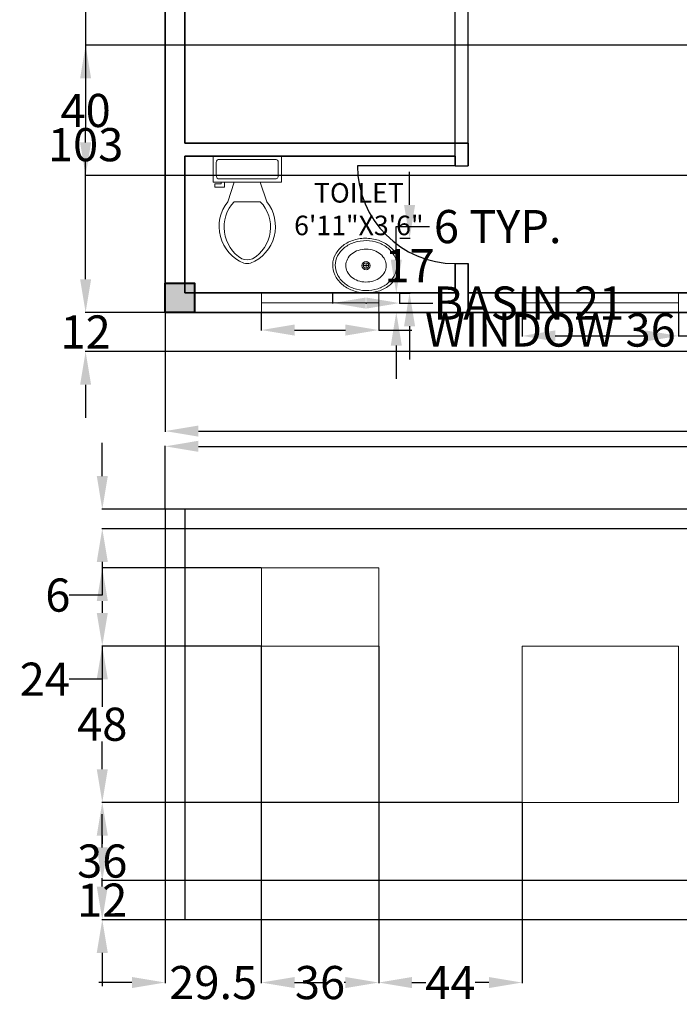
# Model space of a CAD drawing. Units: inches. Extents: x -107 to 647, y -210 to 500.
# Tile 1 of 7: x -20 to 183, y -210 to 92. Entities that reach past the tile are written whole.
import ezdxf

# ---------------------------------------------------------------- set-up
doc = ezdxf.new("R2010")
doc.units = ezdxf.units.IN
doc.header["$MEASUREMENT"] = 0
for name, color, linetype, lineweight in [('A-ANNO-DIMS', 2, 'Continuous', 18), ('A-AREA-IDEN', 7, 'Continuous', 18), ('A-COLS', 7, 'Continuous', 40), ('A-DOOR', 3, 'Continuous', 25), ('A-ELEV', 30, 'Continuous', 25), ('A-ELEV-GLAZ', 4, 'Continuous', 18), ('A-FLOR-FIXT', 9, 'Continuous', 18), ('A-GLAZ', 4, 'Continuous', 18), ('A-WALL', 7, 'Continuous', 35)]:
    doc.layers.add(name, color=color, linetype=linetype, lineweight=lineweight)
doc.styles.get("Standard").update_dxf_attribs({"font": 'arial.ttf'})
doc.dimstyles.get("Standard").update_dxf_attribs({"dimtxt": 10.18, "dimasz": 10.18, "dimexe": 0.18, "dimexo": 0.0625, "dimgap": 0.09, "dimtad": 0, "dimtih": 1, "dimtoh": 1, "dimdec": 0, "dimzin": 0, "dimdsep": 46, "dimlunit": 3, "dimtxsty": 'Standard', "dimcen": 0.09, "dimadec": 0, "dimazin": 0, "dimtfac": 1, "dimtdec": 0, "dimtofl": 0, "dimtmove": 0, "dimatfit": 3, "dimfxl": 1, "dimtolj": 1, "dimtzin": 0, "dimarcsym": 0})

# ---------------------------------------------------------------- blocks, each defined once
blk = doc.blocks.new('Sink - Oval top')
for p, q in [((-1, 0), (1, 0)), ((0, 1), (0, -1))]:
    blk.add_line(p, q)
for points in [[(-12.23, 0.39, 0.117634), (-11.46, -3.36, 0.104469), (-8.88, -6.8, 0.090016), (-5.08, -9.07, 0.08192), (-0.32, -10.02, 0.08192), (4.49, -9.38, 0.090016), (8.42, -7.36, 0.104469), (11.22, -4.09, 0.117634), (12.23, -0.39, 0.117634), (11.46, 3.36, 0.104469), (8.88, 6.8, 0.090016), (5.08, 9.07, 0.08192), (0.32, 10.02, 0.08192), (-4.49, 9.38, 0.090016), (-8.42, 7.36, 0.104469), (-11.22, 4.09, 0.117634)], [(-11.29, 0.16, 0.118622), (-10.52, -3.25, 0.104678), (-8.07, -6.36, 0.089562), (-4.54, -8.37, 0.081185), (-0.13, -9.15, 0.081185), (4.3, -8.49, 0.089562), (7.89, -6.58, 0.104678), (10.42, -3.55, 0.118622), (11.29, -0.16, 0.118622), (10.52, 3.25, 0.104678), (8.07, 6.36, 0.089562), (4.54, 8.37, 0.081185), (0.13, 9.15, 0.081185), (-4.3, 8.49, 0.089562), (-7.89, 6.58, 0.104678), (-10.42, 3.55, 0.118622)], [(-7.42, 0.08, 0.118283), (-6.91, -2.17, 0.104607), (-5.29, -4.21, 0.089718), (-2.97, -5.53, 0.081436), (-0.07, -6.04, 0.081436), (2.84, -5.59, 0.089718), (5.2, -4.33, 0.104607), (6.86, -2.32, 0.118283), (7.42, -0.08, 0.118283), (6.91, 2.17, 0.104607), (5.29, 4.21, 0.089718), (2.97, 5.53, 0.081436), (0.07, 6.04, 0.081436), (-2.84, 5.59, 0.089718), (-5.2, 4.33, 0.104607), (-6.86, 2.32, 0.118283)]]:
    blk.add_lwpolyline(points, format="xyb", close=True)
for radius in [1.5, 1]:
    blk.add_circle((0, 0), radius)
blk = doc.blocks.new('Toilet - top')
for p, q in [((9.5, -6), (9.5, -2)), ((-10, -8.5), (-8, -8.5)), ((-10, -9.5), (-10, -8.5)), ((-8, -8.5), (-8, -8)), ((-7, -8), (-7, -9.5)), ((-4, -8), (-6, -14)), ((4, -8), (6, -14)), ((-7, -9.5), (-10, -9.5)), ((4, -14), (-4, -14))]:
    blk.add_line(p, q)
blk.add_lwpolyline([(10.5, -8), (10.5, 0), (-10.5, 0), (-10.5, -8)], close=True)
for points in [[(-9.5, -2), (-9.5, -6)], [(8.5, -1), (-8.5, -1)], [(-8.5, -7), (8.5, -7)]]:
    blk.add_lwpolyline(points)
for centre, radius, start, end in [((-8.62, -1.88), 0.884, 81.8699, 188.1301), ((8.62, -1.88), 0.884, 351.8699, 98.1301), ((-8.62, -6.12), 0.884, 171.8699, 278.1301), ((8.62, -6.12), 0.884, 261.8699, 8.1301), ((3.52, -21.58), 12.17, 141.4691, 247.9714), ((4.2, -21.82), 11.33, 136.3677, 238.9468), ((-3.52, -21.58), 12.17, 292.0284, 38.5307), ((-4.2, -21.82), 11.33, 301.053, 43.6321), ((0, -27.88), 4, 245.7318, 294.2682), ((0, -29), 4, 254.8605, 285.1395)]:
    blk.add_arc(centre, radius, start, end)
blk = doc.blocks.new('DOOR-SWING-30IN')
for p, q in [((0, 0), (4, 0)), ((0, 0), (-30, 0)), ((0, -30), (4, -30))]:
    blk.add_line(p, q)
blk.add_arc((0, 0), 30, 180, 270)
blk = doc.blocks.new('WINDOW-48IN')
for p, q in [((0, 6), (0, 0)), ((48, 6), (48, 0)), ((0, 3), (48, 3))]:
    blk.add_line(p, q)
blk = doc.blocks.new('WINDOW-36IN')
for p, q in [((0, 6), (0, 0)), ((36, 6), (36, 0)), ((0, 3), (36, 3))]:
    blk.add_line(p, q)
blk = doc.blocks.new('WINDOW-ELEV-48X48IN')
blk.add_lwpolyline([(0, 48), (48, 48), (48, 0), (0, 0)], close=True)
blk = doc.blocks.new('COLUMN-9X9IN')
blk.add_lwpolyline([(0, 9), (9, 9), (9, 0), (0, 0)], close=True)
blk.add_solid([(0, 9), (0, 0), (9, 9), (9, 0)])
blk = doc.blocks.new('*D26')
at = {"layer": 'A-ANNO-DIMS', "color": 0, "lineweight": -2, "transparency": 16777216}
for p, q in [((134.58, 2.26), (134.58, -5.05)), ((182.58, 2.26), (182.58, -5.05)), ((144.76, -4.87), (172.4, -4.87)), ((182.58, -4.87), (192.76, -4.87))]:
    blk.add_line(p, q, dxfattribs=at)
at = {"layer": 'A-ANNO-DIMS', "color": 0, "transparency": 16777216}
for points in [[(144.76, -3.18), (144.76, -6.57), (134.58, -4.87)], [(172.4, -3.18), (172.4, -6.57), (182.58, -4.87)]]:
    blk.add_solid(points, dxfattribs=at)
at = {"layer": 'Defpoints', "color": 0, "transparency": 16777216}
for p in [(134.58, 2.33), (182.58, 2.33), (182.58, -4.87)]:
    blk.add_point(p, dxfattribs=at)
at = {"layer": 'A-ANNO-DIMS', "color": 0, "transparency": 16777216, "insert": (251.01, -4.87), "char_height": 10.18, "attachment_point": 5}
blk.add_mtext('\\A1;WINDOW 48 TYP.', dxfattribs=at)
blk = doc.blocks.new('*D27')
at = {"layer": 'A-ANNO-DIMS', "color": 0, "lineweight": -2, "transparency": 16777216}
for p, q in [((189.78, 18.51), (189.78, 28.69)), ((189.78, 28.69), (199.96, 28.69)), ((182.64, 8.33), (189.96, 8.33)), ((182.64, 2.33), (189.96, 2.33)), ((189.78, -7.85), (189.78, -18.03))]:
    blk.add_line(p, q, dxfattribs=at)
at = {"layer": 'A-ANNO-DIMS', "color": 0, "transparency": 16777216}
for points in [[(188.09, 18.51), (191.48, 18.51), (189.78, 8.33)], [(188.09, -7.85), (191.48, -7.85), (189.78, 2.33)]]:
    blk.add_solid(points, dxfattribs=at)
at = {"layer": 'Defpoints', "color": 0, "transparency": 16777216}
for p in [(182.58, 8.33), (189.78, 8.33), (182.58, 2.33)]:
    blk.add_point(p, dxfattribs=at)
at = {"layer": 'A-ANNO-DIMS', "color": 0, "transparency": 16777216, "insert": (220.9, 28.69), "char_height": 10.18, "attachment_point": 5}
blk.add_mtext('\\A1;6 TYP.', dxfattribs=at)
blk = doc.blocks.new('*D28')
at = {"layer": 'A-ANNO-DIMS', "color": 0, "lineweight": -2, "transparency": 16777216}
for p, q in [((54.58, 2.26), (54.58, -3.25)), ((90.58, 2.26), (90.58, -3.25)), ((64.76, -3.07), (80.4, -3.07)), ((90.58, -3.07), (100.76, -3.07))]:
    blk.add_line(p, q, dxfattribs=at)
at = {"layer": 'A-ANNO-DIMS', "color": 0, "transparency": 16777216}
for points in [[(64.76, -1.38), (64.76, -4.77), (54.58, -3.07)], [(80.4, -1.38), (80.4, -4.77), (90.58, -3.07)]]:
    blk.add_solid(points, dxfattribs=at)
at = {"layer": 'Defpoints', "color": 0, "transparency": 16777216}
for p in [(54.58, 2.33), (90.58, 2.33), (90.58, -3.07)]:
    blk.add_point(p, dxfattribs=at)
at = {"layer": 'A-ANNO-DIMS', "color": 0, "transparency": 16777216, "insert": (159.01, -3.07), "char_height": 10.18, "attachment_point": 5}
blk.add_mtext('\\A1;WINDOW 36 TYP.', dxfattribs=at)
blk = doc.blocks.new('*D29')
at = {"layer": 'A-ANNO-DIMS', "color": 0, "lineweight": -2, "transparency": 16777216}
for p, q in [((95.98, 18.51), (95.98, 28.69)), ((95.98, 28.69), (106.16, 28.69)), ((90.64, 8.33), (96.16, 8.33)), ((90.64, 2.33), (96.16, 2.33)), ((95.98, -7.85), (95.98, -18.03))]:
    blk.add_line(p, q, dxfattribs=at)
at = {"layer": 'A-ANNO-DIMS', "color": 0, "transparency": 16777216}
for points in [[(94.29, 18.51), (97.68, 18.51), (95.98, 8.33)], [(94.29, -7.85), (97.68, -7.85), (95.98, 2.33)]]:
    blk.add_solid(points, dxfattribs=at)
at = {"layer": 'Defpoints', "color": 0, "transparency": 16777216}
for p in [(90.58, 8.33), (95.98, 8.33), (90.58, 2.33)]:
    blk.add_point(p, dxfattribs=at)
at = {"layer": 'A-ANNO-DIMS', "color": 0, "transparency": 16777216, "insert": (127.1, 28.69), "char_height": 10.18, "attachment_point": 5}
blk.add_mtext('\\A1;6 TYP.', dxfattribs=at)
blk = doc.blocks.new('*D36')
at = {"layer": 'A-ANNO-DIMS', "color": 0, "lineweight": -2, "transparency": 16777216}
for p, q in [((76.44, 8.23), (76.44, 5.03)), ((96.98, 8.23), (96.98, 5.03)), ((86.62, 5.21), (86.8, 5.21)), ((96.98, 5.21), (107.16, 5.21))]:
    blk.add_line(p, q, dxfattribs=at)
at = {"layer": 'A-ANNO-DIMS', "color": 0, "transparency": 16777216}
for points in [[(86.62, 6.9), (86.62, 3.51), (76.44, 5.21)], [(86.8, 6.9), (86.8, 3.51), (96.98, 5.21)]]:
    blk.add_solid(points, dxfattribs=at)
at = {"layer": 'Defpoints', "color": 0, "transparency": 16777216}
for p in [(76.44, 8.29), (96.98, 8.29), (96.98, 5.21)]:
    blk.add_point(p, dxfattribs=at)
at = {"layer": 'A-ANNO-DIMS', "color": 0, "transparency": 16777216, "insert": (136.65, 5.21), "char_height": 10.18, "attachment_point": 5}
blk.add_mtext('\\A1;BASIN 21', dxfattribs=at)
blk = doc.blocks.new('*D37')
at = {"layer": 'A-ANNO-DIMS', "color": 0, "lineweight": -2, "transparency": 16777216}
for p, q in [((100.06, 35.32), (100.06, 45.5)), ((97.04, 25.14), (100.24, 25.14)), ((97.04, 8.29), (100.24, 8.29)), ((100.06, -1.89), (100.06, -12.07))]:
    blk.add_line(p, q, dxfattribs=at)
at = {"layer": 'A-ANNO-DIMS', "color": 0, "transparency": 16777216}
for points in [[(98.37, 35.32), (101.76, 35.32), (100.06, 25.14)], [(98.37, -1.89), (101.76, -1.89), (100.06, 8.29)]]:
    blk.add_solid(points, dxfattribs=at)
at = {"layer": 'Defpoints', "color": 0, "transparency": 16777216}
for p in [(96.98, 25.14), (100.06, 25.14), (96.98, 8.29)]:
    blk.add_point(p, dxfattribs=at)
at = {"layer": 'A-ANNO-DIMS', "color": 0, "transparency": 16777216, "insert": (100.06, 16.71), "char_height": 10.18, "attachment_point": 5}
blk.add_mtext('\\A1;17', dxfattribs=at)
blk = doc.blocks.new('*D72')
at = {"layer": 'A-ANNO-DIMS', "color": 0, "lineweight": -2, "transparency": 16777216}
for p, q in [((25.08, 2.26), (25.08, -34.27)), ((409.08, 2.26), (409.08, -34.27)), ((35.26, -34.09), (205.77, -34.09)), ((398.9, -34.09), (228.39, -34.09))]:
    blk.add_line(p, q, dxfattribs=at)
at = {"layer": 'A-ANNO-DIMS', "color": 0, "transparency": 16777216}
for points in [[(35.26, -32.39), (35.26, -35.79), (25.08, -34.09)], [(398.9, -32.39), (398.9, -35.79), (409.08, -34.09)]]:
    blk.add_solid(points, dxfattribs=at)
at = {"layer": 'Defpoints', "color": 0, "transparency": 16777216}
for p in [(25.08, 2.33), (409.08, 2.33), (409.08, -34.09)]:
    blk.add_point(p, dxfattribs=at)
at = {"layer": 'A-ANNO-DIMS', "color": 0, "transparency": 16777216, "insert": (217.08, -34.09), "char_height": 10.18, "attachment_point": 5}
blk.add_mtext('\\A1;384', dxfattribs=at)
blk = doc.blocks.new('*D74')
at = {"layer": 'A-ANNO-DIMS', "color": 0, "lineweight": -2, "transparency": 16777216}
for p, q in [((0.67, 12.51), (0.67, 22.69)), ((203.02, 2.33), (0.49, 2.33)), ((203.02, -9.67), (0.49, -9.67)), ((0.67, -19.85), (0.67, -30.03))]:
    blk.add_line(p, q, dxfattribs=at)
at = {"layer": 'A-ANNO-DIMS', "color": 0, "transparency": 16777216}
for points in [[(-1.03, 12.51), (2.36, 12.51), (0.67, 2.33)], [(-1.03, -19.85), (2.36, -19.85), (0.67, -9.67)]]:
    blk.add_solid(points, dxfattribs=at)
at = {"layer": 'Defpoints', "color": 0, "transparency": 16777216}
for p in [(0.67, 2.33), (203.08, 2.33), (203.08, -9.67)]:
    blk.add_point(p, dxfattribs=at)
at = {"layer": 'A-ANNO-DIMS', "color": 0, "transparency": 16777216, "insert": (0.67, -3.67), "char_height": 10.18, "attachment_point": 5}
blk.add_mtext('\\A1;12', dxfattribs=at)
blk = doc.blocks.new('*D79')
at = {"layer": 'A-ANNO-DIMS', "color": 0, "lineweight": -2, "transparency": 16777216}
for p, q in [((25.02, 105.33), (0.49, 105.33)), ((0.67, 95.15), (0.67, 59.12)), ((0.67, 12.51), (0.67, 48.53)), ((25.02, 2.33), (0.49, 2.33))]:
    blk.add_line(p, q, dxfattribs=at)
at = {"layer": 'A-ANNO-DIMS', "color": 0, "transparency": 16777216}
for points in [[(-1.03, 95.15), (2.36, 95.15), (0.67, 105.33)], [(-1.03, 12.51), (2.36, 12.51), (0.67, 2.33)]]:
    blk.add_solid(points, dxfattribs=at)
at = {"layer": 'Defpoints', "color": 0, "transparency": 16777216}
for p in [(0.67, 105.33), (25.08, 105.33), (25.08, 2.33)]:
    blk.add_point(p, dxfattribs=at)
at = {"layer": 'A-ANNO-DIMS', "color": 0, "transparency": 16777216, "insert": (0.67, 53.83), "char_height": 10.18, "attachment_point": 5}
blk.add_mtext('\\A1;103', dxfattribs=at)
blk = doc.blocks.new('*D80')
at = {"layer": 'A-ANNO-DIMS', "color": 0, "lineweight": -2, "transparency": 16777216}
for p, q in [((367.02, 84.33), (0.49, 84.33)), ((0.67, 74.15), (0.67, 69.61)), ((0.67, 54.51), (0.67, 59.04)), ((367.02, 44.33), (0.49, 44.33))]:
    blk.add_line(p, q, dxfattribs=at)
at = {"layer": 'A-ANNO-DIMS', "color": 0, "transparency": 16777216}
for points in [[(-1.03, 74.15), (2.36, 74.15), (0.67, 84.33)], [(-1.03, 54.51), (2.36, 54.51), (0.67, 44.33)]]:
    blk.add_solid(points, dxfattribs=at)
at = {"layer": 'Defpoints', "color": 0, "transparency": 16777216}
for p in [(0.67, 84.33), (367.08, 84.33), (367.08, 44.33)]:
    blk.add_point(p, dxfattribs=at)
at = {"layer": 'A-ANNO-DIMS', "color": 0, "transparency": 16777216, "insert": (0.67, 64.33), "char_height": 10.18, "attachment_point": 5}
blk.add_mtext('\\A1;40', dxfattribs=at)
blk = doc.blocks.new('*D82')
at = {"layer": 'A-ANNO-DIMS', "color": 0, "lineweight": -2, "transparency": 16777216}
for p, q in [((103.9, 488.74), (93.72, 488.74)), ((114.08, 50.39), (114.08, 488.92)), ((118.08, 54.39), (118.08, 488.92)), ((128.26, 488.74), (138.44, 488.74))]:
    blk.add_line(p, q, dxfattribs=at)
at = {"layer": 'A-ANNO-DIMS', "color": 0, "transparency": 16777216}
for points in [[(103.9, 490.44), (103.9, 487.04), (114.08, 488.74)], [(128.26, 490.44), (128.26, 487.04), (118.08, 488.74)]]:
    blk.add_solid(points, dxfattribs=at)
at = {"layer": 'Defpoints', "color": 0, "transparency": 16777216}
for p in [(118.08, 488.74), (118.08, 54.33), (114.08, 50.33)]:
    blk.add_point(p, dxfattribs=at)
at = {"layer": 'A-ANNO-DIMS', "color": 0, "transparency": 16777216, "insert": (142.05, 488.74), "char_height": 10.18, "attachment_point": 5}
blk.add_mtext('\\A1;4', dxfattribs=at)
blk = doc.blocks.new('*D84')
at = {"layer": 'A-ANNO-DIMS', "color": 0, "lineweight": -2, "transparency": 16777216}
for p, q in [((25.08, -58.01), (25.08, -38.59)), ((35.26, -38.77), (205.77, -38.77)), ((398.9, -38.77), (228.39, -38.77)), ((409.08, -58.01), (409.08, -38.59))]:
    blk.add_line(p, q, dxfattribs=at)
at = {"layer": 'A-ANNO-DIMS', "color": 0, "transparency": 16777216}
for points in [[(35.26, -37.07), (35.26, -40.46), (25.08, -38.77)], [(398.9, -37.07), (398.9, -40.46), (409.08, -38.77)]]:
    blk.add_solid(points, dxfattribs=at)
at = {"layer": 'Defpoints', "color": 0, "transparency": 16777216}
for p in [(409.08, -38.77), (25.08, -58.07), (409.08, -58.07)]:
    blk.add_point(p, dxfattribs=at)
at = {"layer": 'A-ANNO-DIMS', "color": 0, "transparency": 16777216, "insert": (217.08, -38.77), "char_height": 10.18, "attachment_point": 5}
blk.add_mtext('\\A1;384', dxfattribs=at)
blk = doc.blocks.new('*D86')
at = {"layer": 'A-ANNO-DIMS', "color": 0, "lineweight": -2, "transparency": 16777216}
for p, q in [((54.58, -100.13), (54.58, -203.55)), ((25.08, -184.13), (25.08, -203.55)), ((14.9, -203.37), (4.72, -203.37)), ((64.76, -203.37), (74.94, -203.37))]:
    blk.add_line(p, q, dxfattribs=at)
at = {"layer": 'A-ANNO-DIMS', "color": 0, "transparency": 16777216}
for points in [[(14.9, -201.67), (14.9, -205.06), (25.08, -203.37)], [(64.76, -201.67), (64.76, -205.06), (54.58, -203.37)]]:
    blk.add_solid(points, dxfattribs=at)
at = {"layer": 'Defpoints', "color": 0, "transparency": 16777216}
for p in [(54.58, -100.07), (25.08, -184.07), (54.58, -203.37)]:
    blk.add_point(p, dxfattribs=at)
at = {"layer": 'A-ANNO-DIMS', "color": 0, "transparency": 16777216, "insert": (39.83, -203.37), "char_height": 10.18, "attachment_point": 5}
blk.add_mtext('\\A1;29.5', dxfattribs=at)
blk = doc.blocks.new('*D87')
at = {"layer": 'A-ANNO-DIMS', "color": 0, "lineweight": -2, "transparency": 16777216}
for p, q in [((54.58, -100.13), (54.58, -203.55)), ((90.58, -100.13), (90.58, -203.55)), ((64.76, -203.37), (65.21, -203.37)), ((80.4, -203.37), (79.96, -203.37))]:
    blk.add_line(p, q, dxfattribs=at)
at = {"layer": 'A-ANNO-DIMS', "color": 0, "transparency": 16777216}
for points in [[(64.76, -201.67), (64.76, -205.06), (54.58, -203.37)], [(80.4, -201.67), (80.4, -205.06), (90.58, -203.37)]]:
    blk.add_solid(points, dxfattribs=at)
at = {"layer": 'Defpoints', "color": 0, "transparency": 16777216}
for p in [(54.58, -100.07), (90.58, -100.07), (90.58, -203.37)]:
    blk.add_point(p, dxfattribs=at)
at = {"layer": 'A-ANNO-DIMS', "color": 0, "transparency": 16777216, "insert": (72.58, -203.37), "char_height": 10.18, "attachment_point": 5}
blk.add_mtext('\\A1;36', dxfattribs=at)
blk = doc.blocks.new('*D88')
at = {"layer": 'A-ANNO-DIMS', "color": 0, "lineweight": -2, "transparency": 16777216}
for p, q in [((54.52, -76.07), (5.6, -76.07)), ((5.78, -86.25), (5.78, -89.89)), ((54.52, -100.07), (5.6, -100.07)), ((5.78, -100.07), (5.78, -110.25)), ((5.78, -110.25), (-4.4, -110.25))]:
    blk.add_line(p, q, dxfattribs=at)
at = {"layer": 'A-ANNO-DIMS', "color": 0, "transparency": 16777216}
for points in [[(4.09, -86.25), (7.48, -86.25), (5.78, -76.07)], [(4.09, -89.89), (7.48, -89.89), (5.78, -100.07)]]:
    blk.add_solid(points, dxfattribs=at)
at = {"layer": 'Defpoints', "color": 0, "transparency": 16777216}
for p in [(54.58, -76.07), (5.78, -100.07), (54.58, -100.07)]:
    blk.add_point(p, dxfattribs=at)
at = {"layer": 'A-ANNO-DIMS', "color": 0, "transparency": 16777216, "insert": (-11.85, -110.25), "char_height": 10.18, "attachment_point": 5}
blk.add_mtext('\\A1;24', dxfattribs=at)
blk = doc.blocks.new('*D89')
at = {"layer": 'A-ANNO-DIMS', "color": 0, "lineweight": -2, "transparency": 16777216}
for p, q in [((54.52, -100.07), (5.6, -100.07)), ((5.78, -110.25), (5.78, -118.78)), ((5.78, -137.89), (5.78, -129.36)), ((134.52, -148.07), (5.6, -148.07))]:
    blk.add_line(p, q, dxfattribs=at)
at = {"layer": 'A-ANNO-DIMS', "color": 0, "transparency": 16777216}
for points in [[(4.09, -110.25), (7.48, -110.25), (5.78, -100.07)], [(4.09, -137.89), (7.48, -137.89), (5.78, -148.07)]]:
    blk.add_solid(points, dxfattribs=at)
at = {"layer": 'Defpoints', "color": 0, "transparency": 16777216}
for p in [(5.78, -100.07), (54.58, -100.07), (134.58, -148.07)]:
    blk.add_point(p, dxfattribs=at)
at = {"layer": 'A-ANNO-DIMS', "color": 0, "transparency": 16777216, "insert": (5.78, -124.07), "char_height": 10.18, "attachment_point": 5}
blk.add_mtext('\\A1;48', dxfattribs=at)
blk = doc.blocks.new('*D90')
at = {"layer": 'A-ANNO-DIMS', "color": 0, "lineweight": -2, "transparency": 16777216}
for p, q in [((90.58, -100.13), (90.58, -203.55)), ((134.58, -148.13), (134.58, -203.55)), ((100.76, -203.37), (105.02, -203.37)), ((124.4, -203.37), (120.15, -203.37))]:
    blk.add_line(p, q, dxfattribs=at)
at = {"layer": 'A-ANNO-DIMS', "color": 0, "transparency": 16777216}
for points in [[(100.76, -201.67), (100.76, -205.06), (90.58, -203.37)], [(124.4, -201.67), (124.4, -205.06), (134.58, -203.37)]]:
    blk.add_solid(points, dxfattribs=at)
at = {"layer": 'Defpoints', "color": 0, "transparency": 16777216}
for p in [(90.58, -100.07), (134.58, -148.07), (134.58, -203.37)]:
    blk.add_point(p, dxfattribs=at)
at = {"layer": 'A-ANNO-DIMS', "color": 0, "transparency": 16777216, "insert": (112.58, -203.37), "char_height": 10.18, "attachment_point": 5}
blk.add_mtext('\\A1;44', dxfattribs=at)
blk = doc.blocks.new('*D91')
at = {"layer": 'A-ANNO-DIMS', "color": 0, "lineweight": -2, "transparency": 16777216}
for p, q in [((134.52, -148.07), (5.6, -148.07)), ((5.78, -158.25), (5.78, -160.78)), ((5.78, -173.89), (5.78, -171.36)), ((25.02, -184.07), (5.6, -184.07))]:
    blk.add_line(p, q, dxfattribs=at)
at = {"layer": 'A-ANNO-DIMS', "color": 0, "transparency": 16777216}
for points in [[(4.09, -158.25), (7.48, -158.25), (5.78, -148.07)], [(4.09, -173.89), (7.48, -173.89), (5.78, -184.07)]]:
    blk.add_solid(points, dxfattribs=at)
at = {"layer": 'Defpoints', "color": 0, "transparency": 16777216}
for p in [(134.58, -148.07), (5.78, -184.07), (25.08, -184.07)]:
    blk.add_point(p, dxfattribs=at)
at = {"layer": 'A-ANNO-DIMS', "color": 0, "transparency": 16777216, "insert": (5.78, -166.07), "char_height": 10.18, "attachment_point": 5}
blk.add_mtext('\\A1;36', dxfattribs=at)
blk = doc.blocks.new('*D94')
at = {"layer": 'A-ANNO-DIMS', "color": 0, "lineweight": -2, "transparency": 16777216}
for p, q in [((5.78, -47.89), (5.78, -37.71)), ((25.02, -58.07), (5.6, -58.07)), ((25.02, -64.07), (5.6, -64.07)), ((5.78, -74.25), (5.78, -84.43)), ((5.78, -84.43), (-4.4, -84.43))]:
    blk.add_line(p, q, dxfattribs=at)
at = {"layer": 'A-ANNO-DIMS', "color": 0, "transparency": 16777216}
for points in [[(4.09, -47.89), (7.48, -47.89), (5.78, -58.07)], [(4.09, -74.25), (7.48, -74.25), (5.78, -64.07)]]:
    blk.add_solid(points, dxfattribs=at)
at = {"layer": 'Defpoints', "color": 0, "transparency": 16777216}
for p in [(25.08, -58.07), (5.78, -64.07), (25.08, -64.07)]:
    blk.add_point(p, dxfattribs=at)
at = {"layer": 'A-ANNO-DIMS', "color": 0, "transparency": 16777216, "insert": (-7.85, -84.43), "char_height": 10.18, "attachment_point": 5}
blk.add_mtext('\\A1;6', dxfattribs=at)
blk = doc.blocks.new('*D95')
at = {"layer": 'A-ANNO-DIMS', "color": 0, "lineweight": -2, "transparency": 16777216}
for p, q in [((5.78, -161.89), (5.78, -151.71)), ((263.02, -172.07), (5.6, -172.07)), ((263.02, -184.07), (5.6, -184.07)), ((5.78, -194.25), (5.78, -204.43))]:
    blk.add_line(p, q, dxfattribs=at)
at = {"layer": 'A-ANNO-DIMS', "color": 0, "transparency": 16777216}
for points in [[(4.09, -161.89), (7.48, -161.89), (5.78, -172.07)], [(4.09, -194.25), (7.48, -194.25), (5.78, -184.07)]]:
    blk.add_solid(points, dxfattribs=at)
at = {"layer": 'Defpoints', "color": 0, "transparency": 16777216}
for p in [(5.78, -172.07), (263.08, -172.07), (263.08, -184.07)]:
    blk.add_point(p, dxfattribs=at)
at = {"layer": 'A-ANNO-DIMS', "color": 0, "transparency": 16777216, "insert": (5.78, -178.07), "char_height": 10.18, "attachment_point": 5}
blk.add_mtext('\\A1;12', dxfattribs=at)

msp = doc.modelspace()

# ---------------------------------------------------------------- linework, layer by layer
at = {"layer": 'A-ELEV'}
for p, q in [((409.082, -58.068), (25.082, -58.068)), ((25.082, -58.068), (25.082, -184.068)), ((31.082, -58.068), (31.082, -184.068)), ((409.082, -64.068), (25.082, -64.068)), ((409.082, -184.068), (25.082, -184.068))]:
    msp.add_line(p, q, dxfattribs=at)
at = {"layer": 'A-ELEV-GLAZ'}
msp.add_lwpolyline([(54.582, -76.068), (90.582, -76.068), (90.582, -100.068), (54.582, -100.068)], close=True, dxfattribs=at)
at = {"layer": 'A-WALL'}
for p, q in [((31.082, 204.325), (31.082, 54.325)), ((31.082, 54.325), (118.082, 54.325)), ((118.082, 54.325), (118.082, 47.325)), ((31.082, 50.325), (114.082, 50.325)), ((31.082, 50.325), (31.082, 8.325)), ((114.082, 50.325), (114.082, 47.325)), ((114.082, 17.325), (114.082, 8.325)), ((118.082, 17.325), (118.082, 8.325)), ((31.082, 8.325), (114.082, 8.325)), ((118.082, 8.325), (199.082, 8.325)), ((118.082, 8.325), (118.082, 2.325))]:
    msp.add_line(p, q, dxfattribs=at)
msp.add_lwpolyline([(25.082, 2.325), (409.082, 2.325), (409.082, 464.325), (25.082, 464.325)], close=True, dxfattribs=at)

# ---------------------------------------------------------------- block references
at = {"layer": 'A-COLS'}
msp.add_blockref('COLUMN-9X9IN', (25.082, 2.325), dxfattribs=at)
at = {"layer": 'A-DOOR'}
msp.add_blockref('DOOR-SWING-30IN', (114.082, 47.325), dxfattribs=at)
at = {"layer": 'A-ELEV-GLAZ'}
msp.add_blockref('WINDOW-ELEV-48X48IN', (134.582, -148.068), dxfattribs=at)
at = {"layer": 'A-FLOR-FIXT'}
msp.add_blockref('Toilet - top', (50.263, 50.325), dxfattribs=at)
at = {"layer": 'A-FLOR-FIXT', "xscale": 0.8367481713405561, "yscale": 0.8367481713405561, "zscale": 0.8367481713405561}
msp.add_blockref('Sink - Oval top', (86.709, 16.712), dxfattribs=at)
at = {"layer": 'A-GLAZ'}
for name, p in [('WINDOW-36IN', (54.582, 2.325)), ('WINDOW-48IN', (134.582, 2.325))]:
    msp.add_blockref(name, p, dxfattribs=at)

# ---------------------------------------------------------------- texts
at = {"layer": 'A-AREA-IDEN', "insert": (65.337, 42.046), "char_height": 6, "attachment_point": 1}
msp.add_mtext_dynamic_manual_height_columns('\\pxqc;TOILET\\P6\'11"X3\'6"', width=38.32847, gutter_width=1, heights=[0], dxfattribs=at)

# ---------------------------------------------------------------- dimensions: what is measured, and where the dimension line sits
at = {"layer": 'A-ANNO-DIMS'}
for base, p1, p2, override, picture, middle in [((118.082, 488.742), (114.082, 50.325), (118.082, 54.325), {"dimdec": 0, "dimlfac": 1, "dimrnd": 0, "dimzin": 0, "dimdsep": 46, "dimlunit": 2}, '*D82', (142.052, 488.742)), ((409.082, -34.091), (25.082, 2.325), (409.082, 2.325), {"dimdec": 0, "dimlfac": 1, "dimrnd": 0, "dimzin": 0, "dimdsep": 46, "dimlunit": 2}, '*D72', (217.082, -34.091)), ((409.082, -38.768), (25.082, -58.068), (409.082, -58.068), {"dimdec": 0, "dimlfac": 1, "dimrnd": 0, "dimzin": 0, "dimdsep": 46, "dimlunit": 2}, '*D84', (217.082, -38.768)), ((54.582, -203.368), (25.082, -184.068), (54.582, -100.068), {"dimdec": 1, "dimlfac": 1, "dimrnd": 0, "dimzin": 0, "dimdsep": 46, "dimlunit": 2}, '*D86', (39.832, -203.368)), ((90.582, -203.368), (54.582, -100.068), (90.582, -100.068), {"dimdec": 0, "dimlfac": 1, "dimrnd": 0, "dimzin": 0, "dimdsep": 46, "dimlunit": 2}, '*D87', (72.582, -203.368)), ((134.582, -203.368), (90.582, -100.068), (134.582, -148.068), {"dimdec": 0, "dimlfac": 1, "dimrnd": 0, "dimzin": 0, "dimdsep": 46, "dimlunit": 2}, '*D90', (112.582, -203.368))]:
    dim = msp.add_linear_dim(base=base, p1=p1, p2=p2, dimstyle='Standard', override=override, dxfattribs=at)
    dim.commit()
    dim.dimension.update_dxf_attribs({"geometry": picture, "text_midpoint": middle})
for base, p1, p2, picture, middle in [((0.665, 105.325), (25.082, 2.325), (25.082, 105.325), '*D79', (0.665, 53.825)), ((0.665, 84.325), (367.082, 44.325), (367.082, 84.325), '*D80', (0.665, 64.325)), ((100.062, 25.137), (96.981, 8.288), (96.981, 25.137), '*D37', (100.062, 16.712)), ((0.665, 2.325), (203.082, -9.675), (203.082, 2.325), '*D74', (0.665, -3.675)), ((5.782, -64.068), (25.082, -58.068), (25.082, -64.068), '*D94', (-7.849, -84.428)), ((5.782, -100.068), (54.582, -76.068), (54.582, -100.068), '*D88', (-11.846, -110.248)), ((5.782, -100.068), (134.582, -148.068), (54.582, -100.068), '*D89', (5.782, -124.068)), ((5.782, -184.068), (134.582, -148.068), (25.082, -184.068), '*D91', (5.782, -166.068)), ((5.782, -172.068), (263.082, -184.068), (263.082, -172.068), '*D95', (5.782, -178.068))]:
    dim = msp.add_linear_dim(base=base, p1=p1, p2=p2, angle=90, dimstyle='Standard', override={"dimdec": 0, "dimlfac": 1, "dimrnd": 0, "dimzin": 0, "dimdsep": 46, "dimlunit": 2}, dxfattribs=at)
    dim.commit()
    dim.dimension.update_dxf_attribs({"geometry": picture, "text_midpoint": middle})
for base, p1, p2, picture, middle in [((95.982, 8.325), (90.582, 2.325), (90.582, 8.325), '*D29', (127.101, 28.685)), ((189.782, 8.325), (182.582, 2.325), (182.582, 8.325), '*D27', (220.901, 28.685))]:
    dim = msp.add_linear_dim(base=base, p1=p1, p2=p2, angle=90, text='<> TYP.', dimstyle='Standard', override={"dimdec": 0, "dimlfac": 1, "dimrnd": 0, "dimzin": 0, "dimdsep": 46, "dimlunit": 2}, dxfattribs=at)
    dim.commit()
    dim.dimension.update_dxf_attribs({"geometry": picture, "text_midpoint": middle})
for base, p1, p2, text, picture, middle in [((90.582, -3.075), (54.582, 2.325), (90.582, 2.325), 'WINDOW <> TYP.', '*D28', (159.012, -3.075)), ((96.981, 5.206), (76.438, 8.288), (96.981, 8.288), 'BASIN <>', '*D36', (136.648, 5.206)), ((182.582, -4.875), (134.582, 2.325), (182.582, 2.325), 'WINDOW <> TYP.', '*D26', (251.012, -4.875))]:
    dim = msp.add_linear_dim(base=base, p1=p1, p2=p2, text=text, dimstyle='Standard', override={"dimdec": 0, "dimlfac": 1, "dimrnd": 0, "dimzin": 0, "dimdsep": 46, "dimlunit": 2}, dxfattribs=at)
    dim.commit()
    dim.dimension.update_dxf_attribs({"geometry": picture, "text_midpoint": middle})

doc.saveas('drawing.dxf')
